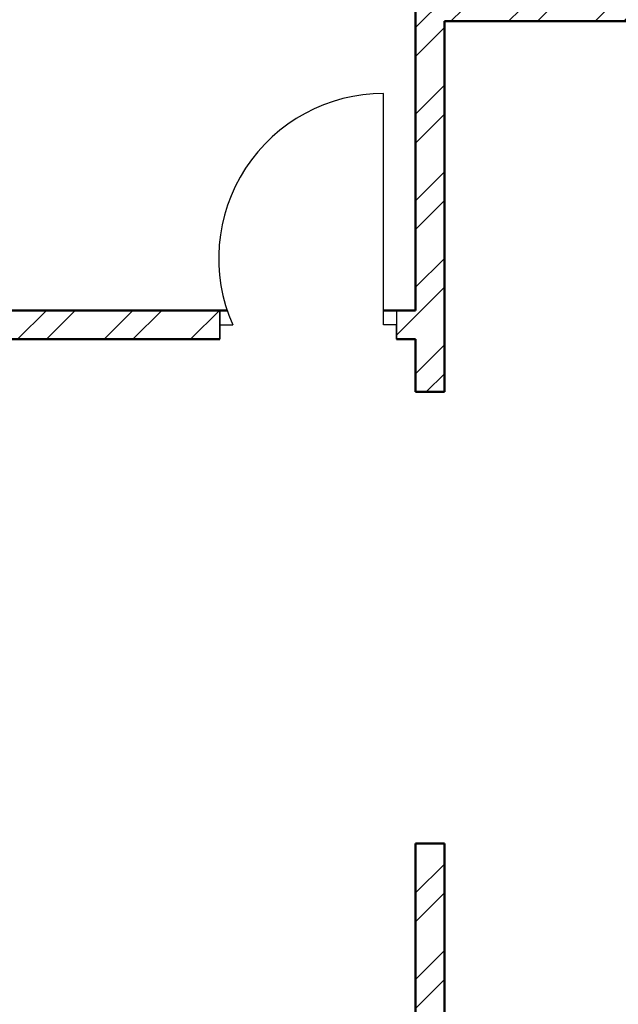
# Model space of a CAD drawing. Units: inches. Extents: x 963 to 2075, y 289 to 2657.
# Tile 17 of 98: x 1310 to 1403, y 1718 to 1872. Entities that reach past the tile are written whole.
import ezdxf

# ---------------------------------------------------------------- set-up
doc = ezdxf.new("R2010")
doc.units = ezdxf.units.IN
for name, color, linetype, lineweight in [('A-DOOR', 4, 'Continuous', 25), ('A-WALL', 7, 'Continuous', 50), ('A-WALL-PATT', 8, 'Continuous', 13)]:
    doc.layers.add(name, color=color, linetype=linetype, lineweight=lineweight)

msp = doc.modelspace()

# ---------------------------------------------------------------- hatches: boundary and pattern name
at = {"layer": 'A-WALL-PATT'}
h = msp.add_hatch(dxfattribs=at)
h.set_pattern_fill('ANSI32', color=256)
h.paths.add_polyline_path([(1296.92, 2558.32), (1203.92, 2558.32), (1203.92, 2493.82), (1191.53, 2493.82), (1191.53, 2489.32), (1211.06, 2489.32), (1211.06, 2492.02), (1211.06, 2493.82), (1208.42, 2493.82), (1208.42, 2553.82), (1292.42, 2553.82), (1292.42, 2538.86), (1296.92, 2538.86)])
h.paths.add_polyline_path([(1442.42, 2558.32), (1349.42, 2558.32), (1349.42, 2538.94), (1353.92, 2538.94), (1353.92, 2553.82), (1437.92, 2553.82), (1437.92, 2493.82), (1434.54, 2493.82), (1434.54, 2489.32), (1448.31, 2489.32), (1448.31, 2491.57), (1448.31, 2493.82), (1442.42, 2493.82)])
h.paths.add_polyline_path([(1415.55, 2491.57), (1415.55, 2493.82), (1340.94, 2493.82), (1340.94, 2489.32), (1371.92, 2489.32), (1371.92, 2378.32), (1367.6, 2378.32), (1367.6, 2373.82), (1371.92, 2373.82), (1371.92, 2355.19), (1376.42, 2355.19), (1376.42, 2489.32), (1415.55, 2489.32)])
h.paths.add_polyline_path([(1304.94, 2491.57), (1304.94, 2493.82), (1296.92, 2493.82), (1296.92, 2514.86), (1292.42, 2514.86), (1292.42, 2493.82), (1232.81, 2493.82), (1232.81, 2489.32), (1256.42, 2489.32), (1256.42, 2327.32), (1253.71, 2327.32), (1253.71, 2322.82), (1328.42, 2322.82), (1328.42, 2331.15), (1323.92, 2331.15), (1323.92, 2327.32), (1260.92, 2327.32), (1260.92, 2373.82), (1323.92, 2373.82), (1323.92, 2357.81), (1328.42, 2357.81), (1328.42, 2373.82), (1346.01, 2373.82), (1346.01, 2376.07), (1346.01, 2378.32), (1260.92, 2378.32), (1260.92, 2489.32), (1304.94, 2489.32)])
h.paths.add_polyline_path([(1226.65, 2327.32), (1124.42, 2327.32), (1124.42, 2347.45), (1119.92, 2347.45), (1119.92, 2322.82), (1163.42, 2322.82), (1163.42, 2305.43), (1165.67, 2305.43), (1167.92, 2305.43), (1167.92, 2322.82), (1226.65, 2322.82), (1226.65, 2325.07)])
h.paths.add_polyline_path([(1095.92, 2489.32), (1124.42, 2489.32), (1131.53, 2489.32), (1131.53, 2491.57), (1131.53, 2493.82), (1119.92, 2493.82), (1091.42, 2493.82), (1091.42, 2417.32), (1095.92, 2417.32), (1119.92, 2417.32), (1119.92, 2407.45), (1124.42, 2407.45), (1124.42, 2421.82), (1095.92, 2421.82)])
h.paths.add_polyline_path([(1512.92, 2558.32), (1508.42, 2558.32), (1508.42, 2493.82), (1503.4, 2493.82), (1503.4, 2489.32), (1508.42, 2489.32), (1508.42, 2327.32), (1376.42, 2327.32), (1376.42, 2330.27), (1371.92, 2330.27), (1371.92, 2298.74), (1376.42, 2298.74), (1376.42, 2322.82), (1508.42, 2322.82), (1508.42, 2165.32), (1504.26, 2165.32), (1504.26, 2160.82), (1508.42, 2160.82), (1508.42, 2108.32), (1512.92, 2108.32), (1512.92, 2160.82), (1516.18, 2160.82), (1516.18, 2163.07), (1516.18, 2165.32), (1512.92, 2165.32), (1512.92, 2322.82), (1644.92, 2322.82), (1644.92, 2298.74), (1649.42, 2298.74), (1649.42, 2322.82), (1649.42, 2330.94), (1647.17, 2330.94), (1644.92, 2330.94), (1644.92, 2327.32), (1512.92, 2327.32), (1512.92, 2489.32), (1516.76, 2489.32), (1516.76, 2491.57), (1516.76, 2493.82), (1512.92, 2493.82)])
h.paths.add_polyline_path([(1671.92, 2558.32), (1578.92, 2558.32), (1578.92, 2493.82), (1573.53, 2493.82), (1573.53, 2489.32), (1586.54, 2489.32), (1586.54, 2491.57), (1586.54, 2493.82), (1583.42, 2493.82), (1583.42, 2553.82), (1667.42, 2553.82), (1667.42, 2541.11), (1671.92, 2541.11)])
h.paths.add_polyline_path([(1681.26, 2493.82), (1671.92, 2493.82), (1671.92, 2517.11), (1667.42, 2517.11), (1667.42, 2493.82), (1610.22, 2493.82), (1610.22, 2489.32), (1644.92, 2489.32), (1644.92, 2357.87), (1649.42, 2357.87), (1649.42, 2373.82), (1652.2, 2373.82), (1652.2, 2375.83), (1652.2, 2378.32), (1649.42, 2378.32), (1649.42, 2489.32), (1681.26, 2489.32), (1681.26, 2491.57)])
h.paths.add_polyline_path([(1821.92, 2558.32), (1728.92, 2558.32), (1728.92, 2541), (1733.42, 2541), (1733.42, 2553.82), (1817.42, 2553.82), (1817.42, 2493.82), (1813.51, 2493.82), (1813.51, 2489.32), (1830.08, 2489.32), (1830.08, 2491.57), (1830.08, 2493.82), (1821.92, 2493.82)])
h.paths.add_polyline_path([(1794.24, 2493.82), (1717.26, 2493.82), (1717.26, 2489.32), (1760.42, 2489.32), (1760.42, 2378.32), (1674.4, 2378.32), (1674.4, 2373.82), (1692.92, 2373.82), (1692.92, 2356.95), (1697.42, 2356.95), (1697.42, 2373.82), (1760.42, 2373.82), (1760.42, 2327.32), (1697.42, 2327.32), (1697.42, 2333.34), (1692.92, 2333.34), (1692.92, 2322.82), (1768.04, 2322.82), (1768.04, 2325.07), (1768.04, 2327.32), (1764.92, 2327.32), (1764.92, 2489.32), (1794.24, 2489.32)])
h.paths.add_polyline_path([(1733.42, 2517), (1728.92, 2517), (1728.92, 2493.82), (1733.42, 2493.82)], flags=17)
h.paths.add_polyline_path([(1929.92, 2493.82), (1890.08, 2493.82), (1890.08, 2489.32), (1896.92, 2489.32), (1925.42, 2489.32), (1925.42, 2421.82), (1896.92, 2421.82), (1896.92, 2408.32), (1901.42, 2408.32), (1901.42, 2417.32), (1925.42, 2417.32), (1929.92, 2417.32)])
h.paths.add_polyline_path([(1901.42, 2348.32), (1896.92, 2348.32), (1896.92, 2327.32), (1800.42, 2327.32), (1800.42, 2322.82), (1853.42, 2322.82), (1853.42, 2309.45), (1857.92, 2309.45), (1857.92, 2322.82), (1901.42, 2322.82)])
h.paths.add_polyline_path([(1857.92, 2249.45), (1853.42, 2249.45), (1853.42, 2214.82), (1686.31, 2214.82), (1686.31, 2210.32), (1853.42, 2210.32), (1853.42, 2202.13), (1857.92, 2202.13), (1857.92, 2210.32)])
h.paths.add_polyline_path([(1857.92, 2142.13), (1853.42, 2142.13), (1853.42, 2115.42), (1841.42, 2115.42), (1841.42, 2088.53), (1841.42, 2046.95), (1845.92, 2046.95), (1845.92, 2110.92), (1905.92, 2110.92), (1905.92, 2092.52), (1910.42, 2092.52), (1910.42, 2115.42), (1857.92, 2115.42)])
h.paths.add_polyline_path([(1532.44, 1482.34), (1573.46, 1482.34), (1573.46, 1501), (1532.44, 1501)], flags=9)
h.paths.add_polyline_path([(1438.66, 1486.3), (1479.68, 1486.3), (1479.68, 1504.96), (1438.66, 1504.96)], flags=9)
h.paths.add_polyline_path([(1411.22, 1365.31), (1659.14, 1365.31), (1659.14, 1402.4), (1411.22, 1402.4)], flags=9)
h.paths.add_polyline_path([(1185.67, 2296.3), (1248.16, 2296.3), (1248.16, 2314.95), (1185.67, 2314.95)], flags=9)
h.paths.add_polyline_path([(1177.31, 2187.35), (1216.15, 2187.35), (1216.15, 2206.01), (1177.31, 2206.01)], flags=9)
h.paths.add_polyline_path([(1295.1, 1602.08), (1328.26, 1602.08), (1328.26, 1620.74), (1295.1, 1620.74)], flags=9)
h.paths.add_polyline_path([(1525.13, 2005.99), (1558.39, 2005.99), (1558.39, 2024.65), (1525.13, 2024.65)], flags=9)
h.paths.add_polyline_path([(1459.61, 1977.13), (1472.19, 1977.13), (1472.19, 1987.43), (1459.61, 1987.43)], flags=9)
h.paths.add_polyline_path([(1467.81, 2053.68), (1480.02, 2053.68), (1480.02, 2063.98), (1467.81, 2063.98)], flags=9)
h.paths.add_polyline_path([(1555.18, 2119.02), (1584.56, 2119.02), (1584.56, 2137.68), (1555.18, 2137.68)], flags=25)
h.paths.add_polyline_path([(1405.39, 2115.29), (1444.48, 2115.29), (1444.48, 2133.95), (1405.39, 2133.95)], flags=25)
h.paths.add_polyline_path([(1698.48, 2004.26), (1727.69, 2004.26), (1727.69, 2022.92), (1698.48, 2022.92)], flags=9)
h.paths.add_polyline_path([(1612.16, 1972.86), (1629.02, 1972.86), (1629.02, 1983.16), (1612.16, 1983.16)], flags=9)
h.paths.add_polyline_path([(1608.29, 2060.04), (1625.15, 2060.04), (1625.15, 2070.34), (1608.29, 2070.34)], flags=9)
h.paths.add_polyline_path([(1527.95, 1684.4), (1566.79, 1684.4), (1566.79, 1703.06), (1527.95, 1703.06)], flags=9)
h.paths.add_polyline_path([(1422.79, 1683.59), (1461.63, 1683.59), (1461.63, 1702.25), (1422.79, 1702.25)], flags=9)
h.paths.add_polyline_path([(1531.26, 1732.46), (1574.01, 1732.46), (1574.01, 1751.12), (1531.26, 1751.12)], flags=9)
h.paths.add_polyline_path([(1402.87, 1732.85), (1439.8, 1732.85), (1439.8, 1751.5), (1402.87, 1751.5)], flags=9)
h.paths.add_polyline_path([(1243.12, 1923.13), (1281.96, 1923.13), (1281.96, 1941.79), (1243.12, 1941.79)], flags=9)
h.paths.add_polyline_path([(1181.75, 1792.27), (1244.24, 1792.27), (1244.24, 1810.93), (1181.75, 1810.93)], flags=9)
h.paths.add_polyline_path([(1265.82, 1670.3), (1316.07, 1670.3), (1316.07, 1688.96), (1265.82, 1688.96)], flags=9)
h.paths.add_polyline_path([(1140.26, 1676.05), (1179.1, 1676.05), (1179.1, 1694.71), (1140.26, 1694.71)], flags=9)
h.paths.add_polyline_path([(1107.49, 1490.89), (1143.37, 1490.89), (1143.37, 1509.55), (1107.49, 1509.55)], flags=9)
h.paths.add_polyline_path([(1217.58, 1483.9), (1246.74, 1483.9), (1246.74, 1502.56), (1217.58, 1502.56)], flags=9)
h.paths.add_polyline_path([(1389.21, 1486.92), (1418.37, 1486.92), (1418.37, 1505.58), (1389.21, 1505.58)], flags=9)
h.paths.add_polyline_path([(1672.21, 1602.08), (1705.37, 1602.08), (1705.37, 1620.74), (1672.21, 1620.74)], flags=9)
h.paths.add_polyline_path([(1752.08, 1522.64), (1781.24, 1522.64), (1781.24, 1541.3), (1752.08, 1541.3)], flags=9)
h.paths.add_polyline_path([(1848.27, 1491.26), (1884.16, 1491.26), (1884.16, 1509.92), (1848.27, 1509.92)], flags=9)
h.paths.add_polyline_path([(1822.47, 1685.62), (1861.31, 1685.62), (1861.31, 1704.28), (1822.47, 1704.28)], flags=9)
h.paths.add_polyline_path([(1713.19, 1672.23), (1763.44, 1672.23), (1763.44, 1690.89), (1713.19, 1690.89)], flags=9)
h.paths.add_polyline_path([(1736.62, 1790.58), (1799.11, 1790.58), (1799.11, 1809.24), (1736.62, 1809.24)], flags=9)
h.paths.add_polyline_path([(1691.49, 1916.36), (1730.33, 1916.36), (1730.33, 1935.01), (1691.49, 1935.01)], flags=9)
h.paths.add_polyline_path([(1764.87, 1973.92), (1794.31, 1973.92), (1794.31, 1992.58), (1764.87, 1992.58)], flags=9)
h.paths.add_polyline_path([(1767.85, 2034.02), (1797.29, 2034.02), (1797.29, 2052.67), (1767.85, 2052.67)], flags=9)
h.paths.add_polyline_path([(1851.59, 2060.33), (1880.75, 2060.33), (1880.75, 2078.99), (1851.59, 2078.99)], flags=25)
h.paths.add_polyline_path([(1688.49, 2086.87), (1727.33, 2086.87), (1727.33, 2105.53), (1688.49, 2105.53)], flags=9)
h.paths.add_polyline_path([(1537.74, 2293.58), (1580.49, 2293.58), (1580.49, 2312.24), (1537.74, 2312.24)], flags=25)
h.paths.add_polyline_path([(1425.59, 2296.11), (1468.34, 2296.11), (1468.34, 2314.77), (1425.59, 2314.77)], flags=25)
h.paths.add_polyline_path([(1278.52, 2004.18), (1307.72, 2004.18), (1307.72, 2022.84), (1278.52, 2022.84)], flags=9)
h.paths.add_polyline_path([(1193.28, 1973.63), (1222.72, 1973.63), (1222.72, 1992.29), (1193.28, 1992.29)], flags=9)
h.paths.add_polyline_path([(1192.41, 2040.58), (1221.84, 2040.58), (1221.84, 2059.23), (1192.41, 2059.23)], flags=9)
h.paths.add_polyline_path([(1130.6, 1951.39), (1159.76, 1951.39), (1159.76, 1970.05), (1130.6, 1970.05)], flags=9)
h.paths.add_polyline_path([(1132.83, 2052.49), (1161.98, 2052.49), (1161.98, 2071.15), (1132.83, 2071.15)], flags=9)
h.paths.add_polyline_path([(1265.13, 2334.62), (1315.38, 2334.62), (1315.38, 2353.28), (1265.13, 2353.28)], flags=25)
h.paths.add_polyline_path([(1136.74, 2330.79), (1175.58, 2330.79), (1175.58, 2349.44), (1136.74, 2349.44)], flags=9)
h.paths.add_polyline_path([(1287.42, 2417.2), (1320.58, 2417.2), (1320.58, 2435.86), (1287.42, 2435.86)], flags=25)
h.paths.add_polyline_path([(1430.99, 2329.16), (1469.83, 2329.16), (1469.83, 2347.82), (1430.99, 2347.82)], flags=25)
h.paths.add_polyline_path([(1525.42, 2329.21), (1564.26, 2329.21), (1564.26, 2347.87), (1525.42, 2347.87)], flags=25)
h.paths.add_polyline_path([(1684.52, 2382.8), (1717.68, 2382.8), (1717.68, 2401.46), (1684.52, 2401.46)], flags=25)
h.paths.add_polyline_path([(1704.81, 2340.29), (1755.05, 2340.29), (1755.05, 2358.95), (1704.81, 2358.95)], flags=25)
h.paths.add_polyline_path([(1694.11, 2287.76), (1756.6, 2287.76), (1756.6, 2306.41), (1694.11, 2306.41)], flags=9)
h.paths.add_polyline_path([(1815.78, 2329.86), (1854.62, 2329.86), (1854.62, 2348.52), (1815.78, 2348.52)], flags=9)
h.paths.add_polyline_path([(1842.87, 2514.26), (1878.76, 2514.26), (1878.76, 2532.91), (1842.87, 2532.91)], flags=9)
h.paths.add_polyline_path([(1769.51, 2531.45), (1798.67, 2531.45), (1798.67, 2550.1), (1769.51, 2550.1)], flags=25)
h.paths.add_polyline_path([(1594.77, 2518.47), (1623.93, 2518.47), (1623.93, 2537.13), (1594.77, 2537.13)], flags=25)
h.paths.add_polyline_path([(1520.72, 2516.18), (1556.61, 2516.18), (1556.61, 2534.84), (1520.72, 2534.84)], flags=25)
h.paths.add_polyline_path([(1464.46, 2516.69), (1500.34, 2516.69), (1500.34, 2535.35), (1464.46, 2535.35)], flags=25)
h.paths.add_polyline_path([(1365.7, 2528.97), (1394.85, 2528.97), (1394.85, 2547.63), (1365.7, 2547.63)], flags=25)
h.paths.add_polyline_path([(1222.84, 2516.23), (1252, 2516.23), (1252, 2534.89), (1222.84, 2534.89)], flags=25)
h.paths.add_polyline_path([(1104.55, 2509.6), (1140.43, 2509.6), (1140.43, 2528.26), (1104.55, 2528.26)], flags=9)
h = msp.add_hatch(dxfattribs=at)
h.set_pattern_fill('ANSI32', color=256)
h.paths.add_polyline_path([(1335.97, 2212.57), (1335.97, 2214.82), (1167.92, 2214.82), (1167.92, 2245.43), (1163.42, 2245.43), (1163.42, 2210.32), (1163.42, 2194.81), (1167.92, 2194.81), (1167.92, 2210.32), (1335.97, 2210.32)])
h.paths.add_polyline_path([(1532.44, 1482.34), (1573.46, 1482.34), (1573.46, 1501), (1532.44, 1501)], flags=9)
h.paths.add_polyline_path([(1438.66, 1486.3), (1479.68, 1486.3), (1479.68, 1504.96), (1438.66, 1504.96)], flags=9)
h.paths.add_polyline_path([(1411.22, 1365.31), (1659.14, 1365.31), (1659.14, 1402.4), (1411.22, 1402.4)], flags=9)
h.paths.add_polyline_path([(1185.67, 2296.3), (1248.16, 2296.3), (1248.16, 2314.95), (1185.67, 2314.95)], flags=9)
h.paths.add_polyline_path([(1177.31, 2187.35), (1216.15, 2187.35), (1216.15, 2206.01), (1177.31, 2206.01)], flags=9)
h.paths.add_polyline_path([(1295.1, 1602.08), (1328.26, 1602.08), (1328.26, 1620.74), (1295.1, 1620.74)], flags=9)
h.paths.add_polyline_path([(1525.13, 2005.99), (1558.39, 2005.99), (1558.39, 2024.65), (1525.13, 2024.65)], flags=9)
h.paths.add_polyline_path([(1459.61, 1977.13), (1472.19, 1977.13), (1472.19, 1987.43), (1459.61, 1987.43)], flags=9)
h.paths.add_polyline_path([(1467.81, 2053.68), (1480.02, 2053.68), (1480.02, 2063.98), (1467.81, 2063.98)], flags=9)
h.paths.add_polyline_path([(1555.18, 2119.02), (1584.56, 2119.02), (1584.56, 2137.68), (1555.18, 2137.68)], flags=9)
h.paths.add_polyline_path([(1405.39, 2115.29), (1444.48, 2115.29), (1444.48, 2133.95), (1405.39, 2133.95)], flags=9)
h.paths.add_polyline_path([(1698.48, 2004.26), (1727.69, 2004.26), (1727.69, 2022.92), (1698.48, 2022.92)], flags=9)
h.paths.add_polyline_path([(1612.16, 1972.86), (1629.02, 1972.86), (1629.02, 1983.16), (1612.16, 1983.16)], flags=9)
h.paths.add_polyline_path([(1608.29, 2060.04), (1625.15, 2060.04), (1625.15, 2070.34), (1608.29, 2070.34)], flags=9)
h.paths.add_polyline_path([(1527.95, 1684.4), (1566.79, 1684.4), (1566.79, 1703.06), (1527.95, 1703.06)], flags=9)
h.paths.add_polyline_path([(1422.79, 1683.59), (1461.63, 1683.59), (1461.63, 1702.25), (1422.79, 1702.25)], flags=9)
h.paths.add_polyline_path([(1531.26, 1732.46), (1574.01, 1732.46), (1574.01, 1751.12), (1531.26, 1751.12)], flags=9)
h.paths.add_polyline_path([(1402.87, 1732.85), (1439.8, 1732.85), (1439.8, 1751.5), (1402.87, 1751.5)], flags=9)
h.paths.add_polyline_path([(1243.12, 1923.13), (1281.96, 1923.13), (1281.96, 1941.79), (1243.12, 1941.79)], flags=9)
h.paths.add_polyline_path([(1181.75, 1792.27), (1244.24, 1792.27), (1244.24, 1810.93), (1181.75, 1810.93)], flags=9)
h.paths.add_polyline_path([(1265.82, 1670.3), (1316.07, 1670.3), (1316.07, 1688.96), (1265.82, 1688.96)], flags=9)
h.paths.add_polyline_path([(1140.26, 1676.05), (1179.1, 1676.05), (1179.1, 1694.71), (1140.26, 1694.71)], flags=9)
h.paths.add_polyline_path([(1107.49, 1490.89), (1143.37, 1490.89), (1143.37, 1509.55), (1107.49, 1509.55)], flags=9)
h.paths.add_polyline_path([(1217.58, 1483.9), (1246.74, 1483.9), (1246.74, 1502.56), (1217.58, 1502.56)], flags=9)
h.paths.add_polyline_path([(1389.21, 1486.92), (1418.37, 1486.92), (1418.37, 1505.58), (1389.21, 1505.58)], flags=9)
h.paths.add_polyline_path([(1672.21, 1602.08), (1705.37, 1602.08), (1705.37, 1620.74), (1672.21, 1620.74)], flags=9)
h.paths.add_polyline_path([(1752.08, 1522.64), (1781.24, 1522.64), (1781.24, 1541.3), (1752.08, 1541.3)], flags=9)
h.paths.add_polyline_path([(1848.27, 1491.26), (1884.16, 1491.26), (1884.16, 1509.92), (1848.27, 1509.92)], flags=9)
h.paths.add_polyline_path([(1822.47, 1685.62), (1861.31, 1685.62), (1861.31, 1704.28), (1822.47, 1704.28)], flags=9)
h.paths.add_polyline_path([(1713.19, 1672.23), (1763.44, 1672.23), (1763.44, 1690.89), (1713.19, 1690.89)], flags=9)
h.paths.add_polyline_path([(1736.62, 1790.58), (1799.11, 1790.58), (1799.11, 1809.24), (1736.62, 1809.24)], flags=9)
h.paths.add_polyline_path([(1691.49, 1916.36), (1730.33, 1916.36), (1730.33, 1935.01), (1691.49, 1935.01)], flags=9)
h.paths.add_polyline_path([(1764.87, 1973.92), (1794.31, 1973.92), (1794.31, 1992.58), (1764.87, 1992.58)], flags=9)
h.paths.add_polyline_path([(1767.85, 2034.02), (1797.29, 2034.02), (1797.29, 2052.67), (1767.85, 2052.67)], flags=9)
h.paths.add_polyline_path([(1851.59, 2060.33), (1880.75, 2060.33), (1880.75, 2078.99), (1851.59, 2078.99)], flags=9)
h.paths.add_polyline_path([(1688.49, 2086.87), (1727.33, 2086.87), (1727.33, 2105.53), (1688.49, 2105.53)], flags=9)
h.paths.add_polyline_path([(1537.74, 2293.58), (1580.49, 2293.58), (1580.49, 2312.24), (1537.74, 2312.24)], flags=9)
h.paths.add_polyline_path([(1425.59, 2296.11), (1468.34, 2296.11), (1468.34, 2314.77), (1425.59, 2314.77)], flags=9)
h.paths.add_polyline_path([(1278.52, 2004.18), (1307.72, 2004.18), (1307.72, 2022.84), (1278.52, 2022.84)], flags=9)
h.paths.add_polyline_path([(1193.28, 1973.63), (1222.72, 1973.63), (1222.72, 1992.29), (1193.28, 1992.29)], flags=9)
h.paths.add_polyline_path([(1192.41, 2040.58), (1221.84, 2040.58), (1221.84, 2059.23), (1192.41, 2059.23)], flags=9)
h.paths.add_polyline_path([(1130.6, 1951.39), (1159.76, 1951.39), (1159.76, 1970.05), (1130.6, 1970.05)], flags=9)
h.paths.add_polyline_path([(1132.83, 2052.49), (1161.98, 2052.49), (1161.98, 2071.15), (1132.83, 2071.15)], flags=9)
h.paths.add_polyline_path([(1265.13, 2334.62), (1315.38, 2334.62), (1315.38, 2353.28), (1265.13, 2353.28)], flags=9)
h.paths.add_polyline_path([(1136.74, 2330.79), (1175.58, 2330.79), (1175.58, 2349.44), (1136.74, 2349.44)], flags=9)
h.paths.add_polyline_path([(1287.42, 2417.2), (1320.58, 2417.2), (1320.58, 2435.86), (1287.42, 2435.86)], flags=9)
h.paths.add_polyline_path([(1430.99, 2329.16), (1469.83, 2329.16), (1469.83, 2347.82), (1430.99, 2347.82)], flags=9)
h.paths.add_polyline_path([(1525.42, 2329.21), (1564.26, 2329.21), (1564.26, 2347.87), (1525.42, 2347.87)], flags=9)
h.paths.add_polyline_path([(1684.52, 2382.8), (1717.68, 2382.8), (1717.68, 2401.46), (1684.52, 2401.46)], flags=9)
h.paths.add_polyline_path([(1704.81, 2340.29), (1755.05, 2340.29), (1755.05, 2358.95), (1704.81, 2358.95)], flags=9)
h.paths.add_polyline_path([(1694.11, 2287.76), (1756.6, 2287.76), (1756.6, 2306.41), (1694.11, 2306.41)], flags=9)
h.paths.add_polyline_path([(1815.78, 2329.86), (1854.62, 2329.86), (1854.62, 2348.52), (1815.78, 2348.52)], flags=9)
h.paths.add_polyline_path([(1842.87, 2514.26), (1878.76, 2514.26), (1878.76, 2532.91), (1842.87, 2532.91)], flags=9)
h.paths.add_polyline_path([(1769.51, 2531.45), (1798.67, 2531.45), (1798.67, 2550.1), (1769.51, 2550.1)], flags=9)
h.paths.add_polyline_path([(1594.77, 2518.47), (1623.93, 2518.47), (1623.93, 2537.13), (1594.77, 2537.13)], flags=9)
h.paths.add_polyline_path([(1520.72, 2516.18), (1556.61, 2516.18), (1556.61, 2534.84), (1520.72, 2534.84)], flags=9)
h.paths.add_polyline_path([(1464.46, 2516.69), (1500.34, 2516.69), (1500.34, 2535.35), (1464.46, 2535.35)], flags=9)
h.paths.add_polyline_path([(1365.7, 2528.97), (1394.85, 2528.97), (1394.85, 2547.63), (1365.7, 2547.63)], flags=9)
h.paths.add_polyline_path([(1222.84, 2516.23), (1252, 2516.23), (1252, 2534.89), (1222.84, 2534.89)], flags=9)
h.paths.add_polyline_path([(1104.55, 2509.6), (1140.43, 2509.6), (1140.43, 2528.26), (1104.55, 2528.26)], flags=9)
h = msp.add_hatch(dxfattribs=at)
h.set_pattern_fill('ANSI32', color=256)
h.paths.add_polyline_path([(1473.61, 2163.07), (1473.61, 2165.32), (1376.42, 2165.32), (1376.42, 2227.98), (1371.92, 2227.98), (1371.92, 2214.82), (1368.41, 2214.82), (1368.41, 2210.32), (1371.92, 2210.32), (1371.92, 2160.82), (1395.92, 2160.82), (1395.92, 2090.32), (1217.34, 2090.32), (1217.34, 2085.82), (1395.92, 2085.82), (1458.92, 2085.82), (1458.92, 2108.32), (1454.42, 2108.32), (1454.42, 2090.32), (1400.42, 2090.32), (1400.42, 2160.82), (1473.61, 2160.82)])
h.paths.add_polyline_path([(1649.42, 2210.32), (1653.23, 2210.32), (1653.23, 2214.82), (1649.42, 2214.82), (1649.42, 2227.98), (1644.92, 2227.98), (1644.92, 2165.32), (1550.1, 2165.32), (1550.1, 2160.82), (1620.92, 2160.82), (1620.92, 2112.82), (1555.45, 2112.82), (1555.45, 2108.32), (1584.33, 2108.32), (1584.33, 2084.92), (1588.83, 2084.92), (1588.83, 2108.32), (1625.42, 2108.32), (1667.95, 2108.32), (1667.95, 2022.67), (1588.83, 2022.67), (1588.83, 2047.41), (1584.33, 2047.41), (1584.33, 1996), (1588.83, 1996), (1588.83, 2018.32), (1667.95, 2018.17), (1667.95, 1928.32), (1625.42, 1928.32), (1625.42, 1923.82), (1672.45, 1923.82), (1672.45, 1928.32), (1672.45, 1946.66), (1785.45, 1946.66), (1785.45, 1951.16), (1743.03, 1951.16), (1743.03, 2017.92), (1841.42, 2017.92), (1841.42, 2014.77), (1845.92, 2014.77), (1845.92, 2017.92), (1905.92, 2017.92), (1905.92, 1987.51), (1910.42, 1987.51), (1910.42, 2022.42), (1910.42, 2068.52), (1905.92, 2068.52), (1905.92, 2022.42), (1845.92, 2022.42), (1845.92, 2025.85), (1843.67, 2025.85), (1841.42, 2025.85), (1841.42, 2022.42), (1743.03, 2022.42), (1743.03, 2084.03), (1768.45, 2084.03), (1785.45, 2084.03), (1785.45, 2088.53), (1672.45, 2088.53), (1672.45, 2112.82), (1667.95, 2112.82), (1625.42, 2112.82), (1625.42, 2160.82), (1649.42, 2160.82)])
h.paths.add_polyline_path([(1672.45, 2084.03), (1738.53, 2084.03), (1738.53, 1951.16), (1672.45, 1951.16)], flags=16)
h.paths.add_polyline_path([(1672.45, 2084.03), (1738.53, 2084.03), (1705.49, 2017.6)], flags=0)
h.paths.add_polyline_path([(1262.77, 2085.82), (1258.27, 2085.82), (1258.27, 2023.28), (1184.42, 2023.28), (1184.42, 2018.78), (1258.27, 2018.78), (1258.27, 1950.82), (1262.77, 1950.82)])
h.paths.add_polyline_path([(1312.27, 2085.82), (1307.77, 2085.82), (1307.77, 1950.82), (1312.27, 1950.82)])
h.paths.add_polyline_path([(1458.92, 1950.82), (1395.92, 1950.82), (1216.57, 1950.82), (1216.57, 1946.32), (1346.42, 1946.32), (1395.92, 1946.32), (1395.92, 1875.82), (1371.92, 1875.82), (1371.92, 1826.32), (1368.93, 1826.32), (1368.93, 1821.82), (1371.92, 1821.82), (1371.92, 1813.62), (1376.42, 1813.62), (1376.42, 1871.32), (1474.5, 1871.32), (1474.5, 1873.57), (1474.5, 1875.82), (1400.42, 1875.82), (1400.42, 1946.32), (1454.42, 1946.32), (1454.42, 1928.32), (1458.92, 1928.32)])
h.paths.add_polyline_path([(1184.42, 2120.78), (1167.92, 2120.78), (1167.92, 2134.81), (1165.67, 2134.81), (1163.42, 2134.81), (1163.42, 2120.78), (1119.92, 2120.78), (1119.92, 2098.1), (1124.42, 2098.1), (1124.42, 2116.28), (1167.92, 2116.28), (1179.92, 2116.28), (1179.92, 2045.92), (1184.42, 2045.92), (1184.42, 2090.32), (1184.42, 2116.28)])
h.paths.add_polyline_path([(1124.42, 2018.78), (1179.92, 2018.78), (1179.92, 2016.29), (1184.42, 2016.29), (1184.42, 2023.28), (1184.42, 2026.59), (1182.17, 2026.59), (1179.92, 2026.59), (1179.92, 2023.28), (1124.42, 2023.28), (1124.42, 2074.1), (1119.92, 2074.1), (1119.92, 2018.78), (1119.92, 1979.63), (1124.42, 1979.63)])
h.paths.add_polyline_path([(1184.42, 1925.78), (1184.42, 1946.32), (1184.42, 1996.07), (1182.17, 1996.07), (1179.92, 1996.07), (1179.92, 1925.78), (1124.42, 1925.78), (1124.42, 1955.63), (1119.92, 1955.5), (1119.92, 1921.28), (1158.92, 1921.28), (1158.92, 1909.98), (1163.42, 1909.98), (1163.42, 1921.28), (1184.42, 1921.28)])
h.paths.add_polyline_path([(1341.45, 1826.32), (1163.42, 1826.32), (1163.42, 1849.98), (1158.92, 1849.98), (1158.92, 1821.82), (1158.92, 1804.03), (1163.42, 1804.03), (1163.42, 1821.82), (1341.45, 1821.82)])
h.paths.add_polyline_path([(1222.98, 1713.82), (1163.42, 1713.82), (1163.42, 1744.03), (1161.17, 1744.03), (1158.92, 1744.03), (1158.92, 1713.82), (1119.92, 1713.82), (1119.92, 1694.65), (1124.42, 1694.65), (1124.42, 1709.32), (1158.92, 1709.32), (1222.98, 1709.32)])
h.paths.add_polyline_path([(1328.42, 1713.82), (1252.04, 1713.82), (1252.04, 1711.57), (1252.04, 1709.32), (1256.42, 1709.32), (1256.42, 1547.32), (1232.94, 1547.32), (1232.94, 1545.07), (1232.94, 1542.82), (1292.42, 1542.82), (1292.42, 1527.63), (1296.92, 1527.63), (1296.92, 1542.82), (1299.46, 1542.82), (1299.46, 1547.32), (1260.92, 1547.32), (1260.92, 1658.32), (1343.66, 1658.32), (1343.66, 1660.57), (1343.66, 1662.82), (1328.42, 1662.82), (1328.42, 1676.59), (1327.4, 1676.59), (1323.92, 1676.59), (1323.92, 1662.82), (1260.92, 1662.82), (1260.92, 1709.32), (1323.92, 1709.32), (1323.92, 1699.85), (1328.42, 1699.85)])
h.paths.add_polyline_path([(1649.42, 1875.82), (1625.42, 1875.82), (1625.42, 1928.32), (1620.92, 1928.32), (1588.83, 1928.32), (1588.83, 1950.59), (1584.33, 1950.59), (1584.33, 1928.32), (1555.45, 1928.32), (1555.45, 1923.82), (1620.92, 1923.82), (1620.92, 1875.82), (1548.95, 1875.82), (1548.95, 1873.57), (1548.95, 1871.32), (1644.92, 1871.32), (1644.92, 1813.62), (1649.42, 1813.62), (1649.42, 1821.82), (1652.04, 1821.82), (1652.04, 1824.07), (1652.04, 1826.32), (1649.42, 1826.32)])
h.paths.add_polyline_path([(1512.92, 1871.32), (1516.48, 1871.32), (1516.48, 1875.82), (1512.92, 1875.82), (1512.92, 1923.82), (1512.92, 1928.32), (1512.92, 1930.83), (1508.42, 1930.83), (1508.42, 1875.82), (1504.41, 1875.82), (1504.41, 1871.32), (1508.42, 1871.32), (1508.42, 1713.82), (1376.42, 1713.82), (1376.42, 1743.32), (1371.92, 1743.32), (1371.92, 1709.32), (1371.92, 1706.01), (1376.42, 1706.01), (1376.42, 1709.32), (1508.42, 1709.32), (1508.42, 1547.32), (1501.87, 1547.32), (1501.87, 1542.82), (1508.42, 1542.82), (1508.42, 1482.82), (1508.42, 1436.32), (1512.92, 1436.32), (1512.92, 1542.82), (1519.32, 1542.82), (1519.32, 1545.07), (1519.32, 1547.32), (1512.92, 1547.32), (1512.92, 1709.32), (1644.92, 1709.32), (1644.92, 1707.55), (1649.42, 1707.55), (1649.42, 1709.32), (1649.42, 1743.32), (1644.92, 1743.32), (1644.92, 1713.82), (1512.92, 1713.82)])
h.paths.add_polyline_path([(1129.88, 1545.07), (1129.88, 1547.32), (1124.42, 1547.32), (1095.92, 1547.32), (1095.92, 1614.82), (1124.42, 1614.82), (1124.42, 1619.32), (1095.92, 1619.32), (1091.42, 1619.32), (1091.42, 1542.82), (1095.92, 1542.82), (1119.92, 1542.82), (1129.88, 1542.82)])
h.paths.add_polyline_path([(1208.42, 1542.82), (1211.74, 1542.82), (1211.74, 1547.32), (1198.85, 1547.32), (1198.85, 1542.82), (1203.92, 1542.82), (1203.92, 1478.32), (1208.42, 1478.32), (1296.92, 1478.32), (1296.92, 1503.63), (1292.42, 1503.63), (1292.42, 1482.82), (1208.42, 1482.82)])
h.paths.add_polyline_path([(1430.42, 1542.82), (1435.7, 1542.82), (1435.7, 1545.07), (1435.7, 1547.32), (1422.66, 1547.32), (1422.66, 1545.07), (1422.66, 1542.82), (1425.92, 1542.82), (1425.92, 1482.86), (1341.92, 1482.86), (1341.92, 1502.73), (1337.42, 1502.73), (1337.42, 1478.36), (1425.92, 1478.36), (1425.92, 1440.82), (1425.92, 1436.32), (1430.42, 1436.32)])
h.paths.add_polyline_path([(1698.48, 2004.26), (1727.69, 2004.26), (1727.69, 2022.92), (1698.48, 2022.92)], flags=8)

# ---------------------------------------------------------------- linework, layer by layer
at = {"layer": 'A-DOOR'}
for p, q in [((1366.93, 1824.07), (1366.93, 1860.07)), ((1341.45, 1826.32), (1341.45, 1821.82)), ((1341.45, 1821.82), (1341.45, 1826.32)), ((1341.45, 1826.32), (1341.45, 1824.07)), ((1368.93, 1826.32), (1368.93, 1821.82)), ((1341.45, 1824.07), (1343.45, 1824.07)), ((1368.93, 1824.07), (1366.93, 1824.07)), ((1368.93, 1821.82), (1368.93, 1824.07))]:
    msp.add_line(p, q, dxfattribs=at)
msp.add_arc((1366.93, 1834.41), 25.66, 90, 203.7695, dxfattribs=at)
at = {"layer": 'A-WALL'}
for p, q in [((1371.92, 1875.82), (1371.92, 1826.32)), ((1376.42, 1871.32), (1376.42, 1813.62)), ((1475.86, 1871.32), (1376.42, 1871.32)), ((1163.42, 1826.32), (1342.58, 1826.32)), ((1366.93, 1826.32), (1371.92, 1826.32)), ((1341.45, 1821.82), (1163.42, 1821.82)), ((1371.92, 1821.82), (1368.93, 1821.82)), ((1371.92, 1821.82), (1371.92, 1813.62)), ((1376.42, 1813.62), (1371.92, 1813.62)), ((1376.42, 1743.32), (1371.92, 1743.32)), ((1371.92, 1743.32), (1371.92, 1709.32)), ((1376.42, 1743.32), (1376.42, 1713.82))]:
    msp.add_line(p, q, dxfattribs=at)

doc.saveas('drawing.dxf')
